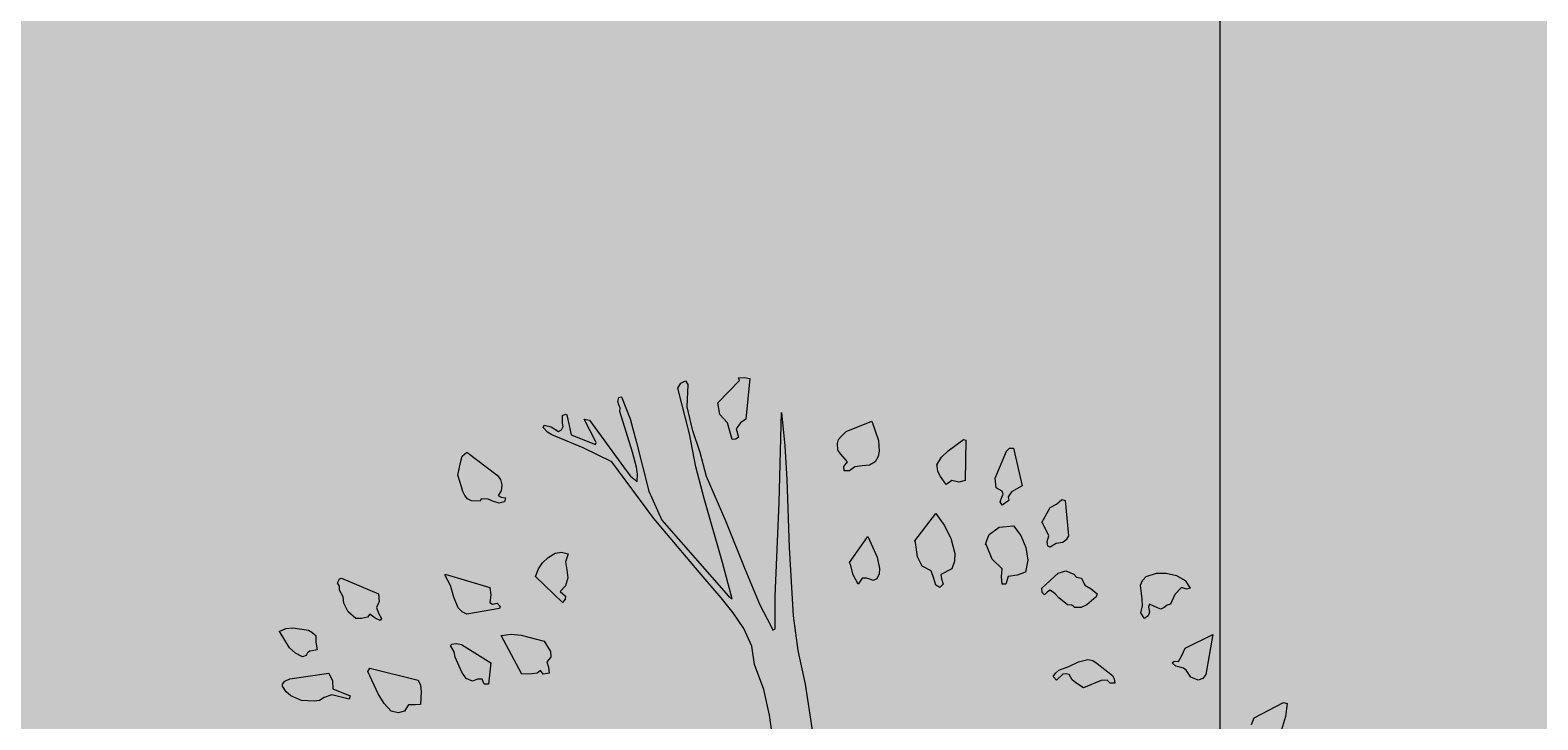
# Model space of a CAD drawing. Units: inches. Extents: x 84 to 1044, y -280 to 906.
# Tile 62 of 105: x 412 to 440, y 748 to 761. Entities that reach past the tile are written whole.
import ezdxf

# ---------------------------------------------------------------- set-up
doc = ezdxf.new("R2010")
doc.units = ezdxf.units.IN
for name, color, linetype, lineweight in [('A-ANNO-DIMS', 2, 'Continuous', 18), ('L-HRDS', 32, 'Continuous', 18), ('L-PLNT', 114, 'Continuous', 15)]:
    doc.layers.add(name, color=color, linetype=linetype, lineweight=lineweight)
doc.layers.add('L-PLNT-PATT', color=9, linetype='Continuous', lineweight=9, true_color=0xafd9aa)
doc.styles.get("Standard").update_dxf_attribs({"font": 'arial.ttf'})
doc.dimstyles.get("Standard").update_dxf_attribs({"dimtxt": 0.18, "dimasz": 0.18, "dimexe": 0.18, "dimexo": 0.0625, "dimgap": 0.09, "dimtad": 0, "dimtih": 1, "dimtoh": 1, "dimdec": 4, "dimzin": 0, "dimdsep": 46, "dimtxsty": 'Standard', "dimcen": 0.09, "dimadec": 0, "dimazin": 0, "dimtfac": 1, "dimtdec": 4, "dimtofl": 0, "dimtmove": 0, "dimatfit": 3, "dimfxl": 1, "dimtolj": 1, "dimtzin": 0, "dimarcsym": 0})

# ---------------------------------------------------------------- blocks, each defined once
blk = doc.blocks.new('A$C37E508DF')
for p, q in [((0.6329, 1.5111), (0.6367, 1.5175)), ((0.6367, 1.5175), (0.6423, 1.5201)), ((0.6423, 1.5201), (0.6453, 1.5158)), ((0.6826, 1.493), (0.7096, 1.5209)), ((0.7083, 1.5239), (0.7152, 1.5244)), ((0.7096, 1.5209), (0.7083, 1.5239)), ((0.7152, 1.5244), (0.7225, 1.5231)), ((0.7225, 1.5231), (0.7174, 1.4729)), ((0.5583, 1.4948), (0.5596, 1.4995)), ((0.5596, 1.4995), (0.563, 1.5003)), ((0.563, 1.5003), (0.5737, 1.4733)), ((0.6475, 1.4545), (0.6329, 1.5111)), ((0.6453, 1.5158), (0.644, 1.4879)), ((0.5596, 1.4905), (0.5583, 1.4948)), ((0.5613, 1.4862), (0.5596, 1.4905)), ((0.5608, 1.4823), (0.5613, 1.4862)), ((0.5767, 1.4317), (0.5608, 1.4823)), ((0.644, 1.4879), (0.6505, 1.46)), ((0.6852, 1.4785), (0.6826, 1.493)), ((0.7589, 1.3691), (0.7615, 1.481)), ((0.7615, 1.481), (0.7658, 1.4395)), ((0.4657, 1.4622), (0.4669, 1.4652)), ((0.4708, 1.4566), (0.4657, 1.4622)), ((0.4669, 1.4652), (0.4755, 1.463)), ((0.4755, 1.463), (0.4845, 1.4575)), ((0.4884, 1.4596), (0.4905, 1.4635)), ((0.4897, 1.4772), (0.4935, 1.4789)), ((0.4897, 1.4678), (0.4897, 1.4772)), ((0.4905, 1.4635), (0.4897, 1.4678)), ((0.4935, 1.4789), (0.4952, 1.478)), ((0.4952, 1.478), (0.5004, 1.4532)), ((0.5313, 1.4437), (0.5167, 1.4729)), ((0.5167, 1.4729), (0.5231, 1.4716)), ((0.5231, 1.4716), (0.5686, 1.409)), ((0.5737, 1.4733), (0.5814, 1.4437)), ((0.6946, 1.4682), (0.6852, 1.4785)), ((0.6976, 1.4579), (0.6946, 1.4682)), ((0.7109, 1.4682), (0.7053, 1.4609)), ((0.7053, 1.4609), (0.7083, 1.4502)), ((0.7174, 1.4729), (0.7109, 1.4682)), ((0.8421, 1.4575), (0.8739, 1.4703)), ((0.8739, 1.4703), (0.882, 1.4463)), ((0.4764, 1.4532), (0.4708, 1.4566)), ((0.5154, 1.4373), (0.4764, 1.4532)), ((0.4845, 1.4575), (0.4884, 1.4596)), ((0.5004, 1.4532), (0.5308, 1.4412)), ((0.5308, 1.4412), (0.5313, 1.4437)), ((0.5814, 1.4437), (0.5969, 1.3833)), ((0.6552, 1.4137), (0.6475, 1.4545)), ((0.6505, 1.46), (0.6603, 1.4317)), ((0.7002, 1.4476), (0.6976, 1.4579)), ((0.7049, 1.448), (0.7002, 1.4476)), ((0.7083, 1.4502), (0.7049, 1.448)), ((0.831, 1.4424), (0.8323, 1.4476)), ((0.8318, 1.4343), (0.831, 1.4424)), ((0.8323, 1.4476), (0.8357, 1.451)), ((0.8357, 1.451), (0.8421, 1.4575)), ((0.882, 1.4463), (0.8829, 1.433)), ((0.9686, 1.4334), (0.9875, 1.4476)), ((0.9875, 1.4476), (0.9905, 1.4467)), ((0.9905, 1.4467), (0.9896, 1.3966)), ((0.3628, 1.4189), (0.3649, 1.4266)), ((0.3649, 1.4266), (0.3709, 1.4317)), ((0.3709, 1.4317), (0.4086, 1.403)), ((0.551, 1.4197), (0.5154, 1.4373)), ((0.5814, 1.4133), (0.5767, 1.4317)), ((0.6603, 1.4317), (0.668, 1.4021)), ((0.7658, 1.4395), (0.7684, 1.3979)), ((0.8353, 1.4292), (0.8318, 1.4343)), ((0.8434, 1.4197), (0.8353, 1.4292)), ((0.8816, 1.4262), (0.8781, 1.4197)), ((0.8829, 1.433), (0.8816, 1.4262)), ((0.9545, 1.4159), (0.9605, 1.4257)), ((0.9605, 1.4257), (0.9686, 1.4334)), ((1.0269, 1.3996), (1.0411, 1.433)), ((1.0411, 1.433), (1.045, 1.4365)), ((1.045, 1.4365), (1.0497, 1.4369)), ((1.0497, 1.4369), (1.0604, 1.3901)), ((0.3598, 1.403), (0.3628, 1.4189)), ((0.6029, 1.3494), (0.551, 1.4197)), ((0.5686, 1.409), (0.5741, 1.4021)), ((0.5827, 1.4043), (0.5814, 1.4133)), ((0.6655, 1.3743), (0.6552, 1.4137)), ((0.8391, 1.4141), (0.8434, 1.4197)), ((0.8395, 1.4086), (0.8391, 1.4141)), ((0.846, 1.4086), (0.8395, 1.4086)), ((0.8528, 1.4137), (0.846, 1.4086)), ((0.8619, 1.4146), (0.8528, 1.4137)), ((0.8709, 1.4154), (0.8619, 1.4146)), ((0.8781, 1.4197), (0.8709, 1.4154)), ((0.9549, 1.4146), (0.9545, 1.4159)), ((0.9558, 1.4077), (0.9549, 1.4146)), ((0.9592, 1.4017), (0.9558, 1.4077)), ((0.3602, 1.4021), (0.3598, 1.403)), ((0.364, 1.3888), (0.3602, 1.4021)), ((0.3657, 1.3828), (0.364, 1.3888)), ((0.4086, 1.403), (0.4125, 1.3979)), ((0.4125, 1.3979), (0.4142, 1.391)), ((0.4142, 1.391), (0.4134, 1.3837)), ((0.5741, 1.4021), (0.5823, 1.3953)), ((0.5823, 1.3953), (0.5827, 1.4043)), ((0.668, 1.4021), (0.6925, 1.3455)), ((0.7684, 1.3979), (0.771, 1.3134)), ((0.966, 1.3914), (0.9592, 1.4017)), ((0.9703, 1.3944), (0.966, 1.3914)), ((0.9733, 1.3966), (0.9703, 1.3944)), ((0.9819, 1.3944), (0.9733, 1.3966)), ((0.9896, 1.3966), (0.9819, 1.3944)), ((1.0282, 1.3876), (1.0269, 1.3996)), ((1.0359, 1.3833), (1.0282, 1.3876)), ((1.0604, 1.3901), (1.0471, 1.3824)), ((0.3683, 1.3781), (0.3657, 1.3828)), ((0.3718, 1.3738), (0.3683, 1.3781)), ((0.3765, 1.3713), (0.3718, 1.3738)), ((0.3872, 1.3708), (0.3765, 1.3713)), ((0.3885, 1.3738), (0.3872, 1.3708)), ((0.3971, 1.3734), (0.3885, 1.3738)), ((0.4039, 1.3704), (0.3971, 1.3734)), ((0.4108, 1.3683), (0.4039, 1.3704)), ((0.4134, 1.3837), (0.4099, 1.3781)), ((0.4099, 1.3781), (0.4134, 1.376)), ((0.4176, 1.37), (0.4108, 1.3683)), ((0.4134, 1.376), (0.4189, 1.3751)), ((0.4189, 1.3751), (0.4176, 1.37)), ((0.5969, 1.3833), (0.6132, 1.3472)), ((0.6882, 1.2949), (0.6655, 1.3743)), ((0.7538, 1.2529), (0.7589, 1.3691)), ((1.0334, 1.37), (1.0351, 1.376)), ((1.0359, 1.3661), (1.0334, 1.37)), ((1.0351, 1.376), (1.0368, 1.3794)), ((1.0368, 1.3794), (1.0359, 1.3833)), ((1.0441, 1.3717), (1.0359, 1.3661)), ((1.0471, 1.3824), (1.0432, 1.3764)), ((1.0432, 1.3764), (1.0441, 1.3717)), ((1.1033, 1.367), (1.1097, 1.373)), ((1.1097, 1.373), (1.114, 1.3717)), ((1.114, 1.3717), (1.1183, 1.328)), ((0.6595, 1.2829), (0.6029, 1.3494)), ((0.9274, 1.3215), (0.9532, 1.3554)), ((0.9532, 1.3554), (0.9635, 1.3413)), ((1.0848, 1.3443), (1.0955, 1.3631)), ((1.0955, 1.3631), (1.1033, 1.367)), ((0.6132, 1.3472), (0.6959, 1.2529)), ((0.6925, 1.3455), (0.7161, 1.2868)), ((0.9635, 1.3413), (0.9721, 1.325)), ((1.0171, 1.3232), (1.0197, 1.3297)), ((1.0197, 1.3297), (1.0321, 1.3387)), ((1.0321, 1.3387), (1.0497, 1.3404)), ((1.0497, 1.3404), (1.0587, 1.3284)), ((1.0861, 1.343), (1.0848, 1.3443)), ((1.0938, 1.328), (1.0861, 1.343)), ((0.771, 1.3134), (0.7761, 1.2285)), ((0.846, 1.2949), (0.8687, 1.3271)), ((0.8687, 1.3271), (0.8803, 1.3014)), ((0.9279, 1.3194), (0.9274, 1.3215)), ((0.9305, 1.3018), (0.9279, 1.3194)), ((0.9721, 1.325), (0.9768, 1.3061)), ((1.0149, 1.3172), (1.0171, 1.3232)), ((1.0162, 1.3164), (1.0149, 1.3172)), ((1.0231, 1.2988), (1.0162, 1.3164)), ((1.0587, 1.3284), (1.0651, 1.3134)), ((1.0651, 1.3134), (1.0677, 1.2975)), ((1.0917, 1.3207), (1.0938, 1.328)), ((1.0925, 1.3151), (1.0917, 1.3207)), ((1.0955, 1.3138), (1.0925, 1.3151)), ((1.1028, 1.3185), (1.0955, 1.3138)), ((1.111, 1.3194), (1.1028, 1.3185)), ((1.1153, 1.3228), (1.111, 1.3194)), ((1.1183, 1.328), (1.1153, 1.3228)), ((0.4597, 1.2868), (0.4648, 1.2945)), ((0.4648, 1.2945), (0.4717, 1.3009)), ((0.4717, 1.3009), (0.4807, 1.3065)), ((0.4807, 1.3065), (0.4884, 1.3074)), ((0.4884, 1.3074), (0.4965, 1.3057)), ((0.4965, 1.3057), (0.4935, 1.2954)), ((0.4935, 1.2954), (0.4948, 1.2855)), ((0.7002, 1.2495), (0.6882, 1.2949)), ((0.8473, 1.2924), (0.846, 1.2949)), ((0.8507, 1.2795), (0.8473, 1.2924)), ((0.8803, 1.3014), (0.8833, 1.2872)), ((0.9365, 1.2902), (0.9305, 1.3018)), ((0.9763, 1.2962), (0.9733, 1.2868)), ((0.9768, 1.3061), (0.9763, 1.2962)), ((1.0359, 1.2868), (1.0231, 1.2988)), ((1.0677, 1.2975), (1.0647, 1.2829)), ((0.2101, 1.2696), (0.2127, 1.2744)), ((0.2127, 1.2744), (0.2152, 1.2752)), ((0.2152, 1.2752), (0.2611, 1.2559)), ((0.3439, 1.2804), (0.3992, 1.2636)), ((0.3439, 1.2787), (0.3439, 1.2804)), ((0.3507, 1.2662), (0.3439, 1.2787)), ((0.4562, 1.2774), (0.4597, 1.2868)), ((0.4897, 1.2452), (0.4562, 1.2774)), ((0.4961, 1.2756), (0.4935, 1.2658)), ((0.4948, 1.2855), (0.4961, 1.2756)), ((0.6865, 1.2508), (0.6595, 1.2829)), ((0.7161, 1.2868), (0.7349, 1.2422)), ((0.8567, 1.2679), (0.8507, 1.2795)), ((0.8619, 1.2752), (0.8567, 1.2679)), ((0.867, 1.2752), (0.8619, 1.2752)), ((0.8713, 1.2739), (0.867, 1.2752)), ((0.8756, 1.2726), (0.8713, 1.2739)), ((0.8799, 1.2744), (0.8756, 1.2726)), ((0.8829, 1.2808), (0.8799, 1.2744)), ((0.8833, 1.2872), (0.8829, 1.2808)), ((0.9476, 1.2842), (0.9365, 1.2902)), ((0.951, 1.2748), (0.9476, 1.2842)), ((0.9532, 1.2666), (0.951, 1.2748)), ((0.9733, 1.2868), (0.9596, 1.2799)), ((0.9596, 1.2799), (0.9605, 1.2744)), ((0.9605, 1.2744), (0.9626, 1.2679)), ((1.0347, 1.2769), (1.0359, 1.2868)), ((1.0359, 1.2679), (1.0347, 1.2769)), ((1.0432, 1.2774), (1.0402, 1.2679)), ((1.0544, 1.2791), (1.0432, 1.2774)), ((1.0647, 1.2829), (1.0544, 1.2791)), ((1.0848, 1.2628), (1.1054, 1.2817)), ((1.1054, 1.2817), (1.1148, 1.2842)), ((1.1148, 1.2842), (1.1247, 1.2804)), ((1.1247, 1.2804), (1.1281, 1.2765)), ((1.1281, 1.2765), (1.1341, 1.2752)), ((1.1341, 1.2752), (1.1384, 1.2666)), ((1.21, 1.2726), (1.2147, 1.2774)), ((1.2147, 1.2774), (1.2276, 1.2817)), ((1.2276, 1.2817), (1.2392, 1.2817)), ((1.2392, 1.2817), (1.2521, 1.2787)), ((1.2521, 1.2787), (1.2632, 1.2722)), ((0.2127, 1.2654), (0.2101, 1.2696)), ((0.2127, 1.2602), (0.2127, 1.2654)), ((0.2174, 1.2521), (0.2127, 1.2602)), ((0.2611, 1.2559), (0.262, 1.2465)), ((0.3546, 1.2516), (0.3507, 1.2662)), ((0.3992, 1.2636), (0.4005, 1.2546)), ((0.4935, 1.2658), (0.4867, 1.2589)), ((0.4867, 1.2589), (0.4935, 1.2529)), ((0.9583, 1.2636), (0.9532, 1.2666)), ((0.9626, 1.2679), (0.9583, 1.2636)), ((1.0402, 1.2679), (1.0359, 1.2679)), ((1.0852, 1.2576), (1.0848, 1.2628)), ((1.0883, 1.2546), (1.0852, 1.2576)), ((1.0921, 1.2585), (1.0883, 1.2546)), ((1.0955, 1.2602), (1.0921, 1.2585)), ((1.1015, 1.2559), (1.0955, 1.2602)), ((1.1063, 1.2508), (1.1015, 1.2559)), ((1.1384, 1.2666), (1.1461, 1.2619)), ((1.1461, 1.2619), (1.1539, 1.2559)), ((1.1539, 1.2559), (1.1526, 1.2521)), ((1.2075, 1.2666), (1.21, 1.2726)), ((1.2096, 1.2491), (1.2075, 1.2666)), ((1.2503, 1.2551), (1.2448, 1.2431)), ((1.2585, 1.2636), (1.2503, 1.2551)), ((1.2645, 1.2615), (1.2585, 1.2636)), ((1.2632, 1.2722), (1.2692, 1.2628)), ((1.2692, 1.2628), (1.2645, 1.2615)), ((0.2182, 1.2443), (0.2174, 1.2521)), ((0.2234, 1.2336), (0.2182, 1.2443)), ((0.262, 1.2465), (0.2586, 1.2388)), ((0.2586, 1.2388), (0.2611, 1.2319)), ((0.3602, 1.2383), (0.3546, 1.2516)), ((0.3649, 1.2336), (0.3602, 1.2383)), ((0.4112, 1.2375), (0.3709, 1.2306)), ((0.4005, 1.2546), (0.3992, 1.2452)), ((0.3992, 1.2452), (0.4026, 1.2431)), ((0.4026, 1.2431), (0.4086, 1.2443)), ((0.4086, 1.2443), (0.4121, 1.2401)), ((0.4121, 1.2401), (0.4112, 1.2375)), ((0.4931, 1.2491), (0.4897, 1.2452)), ((0.4935, 1.2529), (0.4931, 1.2491)), ((0.7015, 1.2323), (0.6865, 1.2508)), ((0.6959, 1.2529), (0.7002, 1.2495)), ((0.7349, 1.2422), (0.7482, 1.216)), ((0.7538, 1.2122), (0.7538, 1.2529)), ((1.117, 1.2422), (1.1063, 1.2508)), ((1.1221, 1.2418), (1.117, 1.2422)), ((1.126, 1.2388), (1.1221, 1.2418)), ((1.1337, 1.2388), (1.126, 1.2388)), ((1.141, 1.2422), (1.1337, 1.2388)), ((1.1526, 1.2521), (1.141, 1.2422)), ((1.2079, 1.2323), (1.21, 1.2409)), ((1.21, 1.2409), (1.2096, 1.2491)), ((1.2186, 1.2431), (1.2173, 1.2392)), ((1.2173, 1.2392), (1.2186, 1.2332)), ((1.2285, 1.2383), (1.2186, 1.2431)), ((1.2328, 1.2366), (1.2285, 1.2383)), ((1.2371, 1.2388), (1.2328, 1.2366)), ((1.2405, 1.2418), (1.2371, 1.2388)), ((1.2448, 1.2431), (1.2405, 1.2418)), ((0.2328, 1.2251), (0.2234, 1.2336)), ((0.2401, 1.2251), (0.2328, 1.2251)), ((0.2474, 1.2268), (0.2401, 1.2251)), ((0.2504, 1.2306), (0.2474, 1.2268)), ((0.2568, 1.2255), (0.2504, 1.2306)), ((0.2633, 1.2229), (0.2568, 1.2255)), ((0.2611, 1.2319), (0.265, 1.2251)), ((0.265, 1.2251), (0.2633, 1.2229)), ((0.3709, 1.2306), (0.3649, 1.2336)), ((0.7148, 1.2126), (0.7015, 1.2323)), ((0.7761, 1.2285), (0.7821, 1.1856)), ((1.2126, 1.2251), (1.2079, 1.2323)), ((1.2169, 1.2285), (1.2126, 1.2251)), ((1.2186, 1.2332), (1.2169, 1.2285)), ((0.1376, 1.2092), (0.1458, 1.2126)), ((0.1389, 1.2079), (0.1376, 1.2092)), ((0.1505, 1.189), (0.1389, 1.2079)), ((0.1458, 1.2126), (0.1548, 1.2135)), ((0.1548, 1.2135), (0.1741, 1.2109)), ((0.1741, 1.2109), (0.1784, 1.2083)), ((0.1784, 1.2083), (0.1831, 1.204)), ((0.1831, 1.204), (0.1831, 1.1959)), ((0.4134, 1.204), (0.4258, 1.2058)), ((0.4391, 1.156), (0.4134, 1.204)), ((0.4258, 1.2058), (0.4382, 1.2045)), ((0.4382, 1.2045), (0.4669, 1.1972)), ((0.7246, 1.1908), (0.7148, 1.2126)), ((0.7482, 1.216), (0.7508, 1.2109)), ((0.7508, 1.2109), (0.7538, 1.2122)), ((1.2628, 1.1882), (1.2975, 1.2053)), ((1.2975, 1.2053), (1.2885, 1.1556)), ((0.1582, 1.1822), (0.1505, 1.189)), ((0.1668, 1.1775), (0.1582, 1.1822)), ((0.1728, 1.1826), (0.1711, 1.1792)), ((0.1758, 1.1847), (0.1728, 1.1826)), ((0.1788, 1.1852), (0.1758, 1.1847)), ((0.1848, 1.1865), (0.1788, 1.1852)), ((0.1831, 1.1959), (0.1848, 1.1865)), ((0.3507, 1.1916), (0.352, 1.1933)), ((0.355, 1.1839), (0.3507, 1.1916)), ((0.352, 1.1933), (0.3576, 1.1942)), ((0.3563, 1.177), (0.355, 1.1839)), ((0.3576, 1.1942), (0.364, 1.1929)), ((0.364, 1.1929), (0.4005, 1.1702)), ((0.4669, 1.1972), (0.4747, 1.1843)), ((0.4747, 1.1843), (0.4751, 1.177)), ((0.7281, 1.168), (0.7246, 1.1908)), ((0.7821, 1.1856), (0.7911, 1.1436)), ((1.2589, 1.1792), (1.2628, 1.1882)), ((0.1711, 1.1792), (0.1668, 1.1775)), ((0.2478, 1.1594), (0.2504, 1.1637)), ((0.2504, 1.1637), (0.3104, 1.1487)), ((0.3645, 1.1586), (0.3563, 1.177)), ((0.4005, 1.1702), (0.3979, 1.1436)), ((0.4751, 1.177), (0.47, 1.1714)), ((0.47, 1.1714), (0.4721, 1.1646)), ((0.4721, 1.1646), (0.473, 1.1573)), ((0.7396, 1.1371), (0.7281, 1.168)), ((1.102, 1.1573), (1.1063, 1.1612)), ((1.1063, 1.1612), (1.1187, 1.1655)), ((1.1187, 1.1655), (1.1307, 1.1714)), ((1.1307, 1.1714), (1.1423, 1.1744)), ((1.1423, 1.1744), (1.1483, 1.1732)), ((1.1483, 1.1732), (1.1539, 1.1693)), ((1.1539, 1.1693), (1.1727, 1.1543)), ((1.2469, 1.1702), (1.2495, 1.1723)), ((1.2478, 1.1693), (1.2469, 1.1702)), ((1.2516, 1.1659), (1.2478, 1.1693)), ((1.2495, 1.1723), (1.2546, 1.1719)), ((1.2563, 1.1646), (1.2516, 1.1659)), ((1.2546, 1.1719), (1.2589, 1.1792)), ((1.2611, 1.1637), (1.2563, 1.1646)), ((1.2641, 1.1612), (1.2611, 1.1637)), ((1.2701, 1.1522), (1.2641, 1.1612)), ((0.1419, 1.1436), (0.1449, 1.1474)), ((0.1419, 1.141), (0.1419, 1.1436)), ((0.1449, 1.1474), (0.1509, 1.1504)), ((0.1509, 1.1504), (0.1994, 1.1573)), ((0.1994, 1.1573), (0.2041, 1.1479)), ((0.2041, 1.1479), (0.2045, 1.138)), ((0.2607, 1.1316), (0.2478, 1.1594)), ((0.3104, 1.1487), (0.3134, 1.1423)), ((0.37, 1.1509), (0.3645, 1.1586)), ((0.3778, 1.1474), (0.37, 1.1509)), ((0.3842, 1.15), (0.3778, 1.1474)), ((0.3898, 1.15), (0.3842, 1.15)), ((0.3923, 1.1436), (0.3898, 1.15)), ((0.3979, 1.1436), (0.3923, 1.1436)), ((0.4519, 1.1564), (0.4391, 1.156)), ((0.458, 1.1573), (0.4519, 1.1564)), ((0.4622, 1.1607), (0.458, 1.1573)), ((0.4657, 1.156), (0.4622, 1.1607)), ((0.473, 1.1573), (0.4657, 1.156)), ((0.7911, 1.1436), (0.8027, 1.0677)), ((1.099, 1.153), (1.102, 1.1573)), ((1.1033, 1.1487), (1.099, 1.153)), ((1.111, 1.156), (1.1033, 1.1487)), ((1.1153, 1.1564), (1.111, 1.156)), ((1.1191, 1.1556), (1.1153, 1.1564)), ((1.1226, 1.1492), (1.1191, 1.1556)), ((1.1273, 1.1453), (1.1226, 1.1492)), ((1.1367, 1.1393), (1.1273, 1.1453)), ((1.1517, 1.1453), (1.1367, 1.1393)), ((1.1586, 1.1483), (1.1517, 1.1453)), ((1.1663, 1.1487), (1.1586, 1.1483)), ((1.1697, 1.1449), (1.1663, 1.1487)), ((1.1757, 1.1449), (1.1697, 1.1449)), ((1.1727, 1.1543), (1.1749, 1.1504)), ((1.1749, 1.1504), (1.1757, 1.1449)), ((1.2791, 1.1487), (1.2701, 1.1522)), ((1.2851, 1.1509), (1.2791, 1.1487)), ((1.2885, 1.1556), (1.2851, 1.1509)), ((0.1462, 1.1342), (0.1419, 1.141)), ((0.1522, 1.1294), (0.1462, 1.1342)), ((0.1655, 1.1234), (0.1522, 1.1294)), ((0.1938, 1.1273), (0.1878, 1.1234)), ((0.2032, 1.1303), (0.1938, 1.1273)), ((0.2247, 1.1251), (0.2032, 1.1303)), ((0.2045, 1.138), (0.226, 1.129)), ((0.226, 1.129), (0.2247, 1.1251)), ((0.268, 1.1196), (0.2607, 1.1316)), ((0.3134, 1.1423), (0.3139, 1.1346)), ((0.3139, 1.1346), (0.3134, 1.1183)), ((0.7469, 1.1054), (0.7396, 1.1371)), ((0.181, 1.1226), (0.1655, 1.1234)), ((0.1878, 1.1234), (0.181, 1.1226)), ((0.277, 1.1101), (0.268, 1.1196)), ((0.2856, 1.108), (0.277, 1.1101)), ((0.2933, 1.1101), (0.2856, 1.108)), ((0.2959, 1.1144), (0.2933, 1.1101)), ((0.2984, 1.1179), (0.2959, 1.1144)), ((0.3066, 1.1179), (0.2984, 1.1179)), ((0.3134, 1.1183), (0.3066, 1.1179)), ((0.7512, 1.0728), (0.7469, 1.1054)), ((1.3485, 1.102), (1.385, 1.1209)), ((1.385, 1.1209), (1.3897, 1.1196)), ((1.3897, 1.1196), (1.3875, 1.1037)), ((1.3455, 1.0934), (1.3485, 1.102)), ((1.3875, 1.1037), (1.3828, 1.087))]:
    blk.add_line(p, q)
blk = doc.blocks.new('*D62')
at = {"layer": 'A-ANNO-DIMS', "color": 0, "lineweight": -2, "transparency": 16777216}
for p, q in [((203.179, 709.183), (203.179, 905.9)), ((896.074, 400.183), (896.074, 905.9)), ((203.359, 905.72), (549.232, 905.72)), ((895.894, 905.72), (550.021, 905.72))]:
    blk.add_line(p, q, dxfattribs=at)
at = {"layer": 'A-ANNO-DIMS', "color": 0, "transparency": 16777216}
for points in [[(203.359, 905.75), (203.359, 905.69), (203.179, 905.72)], [(895.894, 905.75), (895.894, 905.69), (896.074, 905.72)]]:
    blk.add_solid(points, dxfattribs=at)
at = {"layer": 'Defpoints', "color": 0, "transparency": 16777216}
for p in [(896.074, 905.72), (203.179, 709.12), (896.074, 400.12)]:
    blk.add_point(p, dxfattribs=at)
at = {"layer": 'A-ANNO-DIMS', "color": 0, "transparency": 16777216, "insert": (549.627, 905.72), "char_height": 0.18, "attachment_point": 5}
blk.add_mtext('\\A1;692.9', dxfattribs=at)

msp = doc.modelspace()

# ---------------------------------------------------------------- hatches: boundary and pattern name
at = {"layer": 'L-PLNT-PATT', "transparency": 33554597}
h = msp.add_hatch(color=256, dxfattribs=at)
h.dxf.hatch_style = 1
h.paths.add_polyline_path([(434.074, 769.12), (386.074, 769.12), (386.074, 709.12), (434.074, 709.12)])
h.paths.add_polyline_path([(896.074, 847.12), (434.074, 847.12), (434.074, 769.12), (434.074, 709.12), (470.074, 709.12), (506.074, 709.12), (572.074, 709.12), (608.074, 709.12), (698.074, 709.12), (770.074, 709.12), (833.074, 709.12), (896.074, 709.12)])
h.paths.add_polyline_path([(983.074, 847.12), (896.074, 847.12), (896.074, 709.12), (896.074, 547.12), (932.074, 547.12), (983.074, 547.12)])
h.paths.add_polyline_path([(983.074, 547.12), (932.074, 547.12), (932.074, 265.12), (983.074, 265.12)])
h.paths.add_polyline_path([(203.179, 646.12), (203.179, 709.12), (203.179, 745.12), (143.179, 745.12), (143.179, 271.12), (203.179, 271.12), (203.179, 274.12), (203.179, 310.12), (203.179, 574.12)])

# ---------------------------------------------------------------- linework, layer by layer
at = {"layer": 'L-HRDS'}
msp.add_line((434.074, 769.12), (434.074, 709.12), dxfattribs=at)

# ---------------------------------------------------------------- block references
at = {"layer": 'L-PLNT', "xscale": 15.19586232982809, "yscale": 15.19586232982809, "zscale": 15.19586232982809}
msp.add_blockref('A$C37E508DF', (414.225, 731.356), dxfattribs=at)

# ---------------------------------------------------------------- dimensions: what is measured, and where the dimension line sits
at = {"layer": 'A-ANNO-DIMS'}
dim = msp.add_linear_dim(base=(896.074, 905.72), p1=(203.179, 709.12), p2=(896.074, 400.12), dimstyle='Standard', override={"dimdec": 1, "dimlfac": 1, "dimrnd": 0, "dimzin": 0, "dimdsep": 46, "dimlunit": 2}, dxfattribs=at)
dim.commit()
dim.dimension.update_dxf_attribs({"geometry": '*D62', "text_midpoint": (549.627, 905.72)})

doc.saveas('drawing.dxf')
